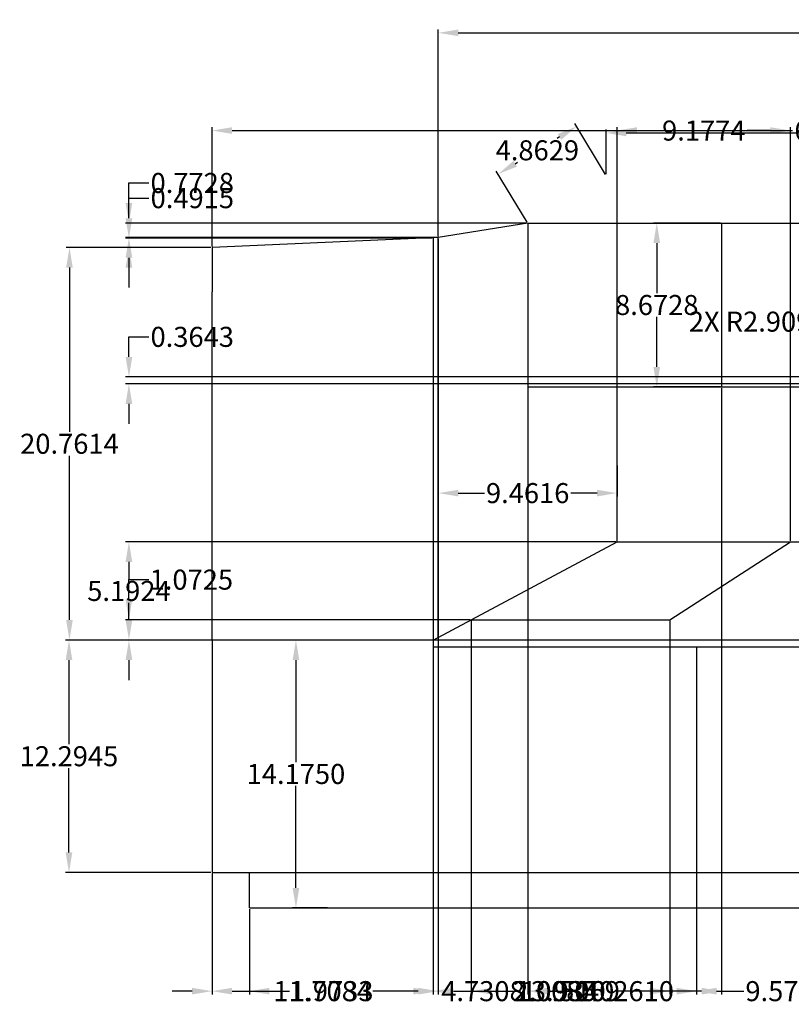
# Model space of a CAD drawing. Units: inches. Extents: x 32.3 to 119.3, y 11.9 to 64.
# Tile 1 of 3: x 32.3 to 73.2, y 11.9 to 64. Entities that reach past the tile are written whole.
import ezdxf

# ---------------------------------------------------------------- set-up
doc = ezdxf.new("R2010")
doc.units = ezdxf.units.IN
doc.header["$MEASUREMENT"] = 0
doc.layers.add('A-ANNO-DIMS', color=2, linetype='Continuous', lineweight=18)
doc.layers.add('A-FURN', color=7, linetype='Continuous', lineweight=25)
doc.styles.get("Standard").update_dxf_attribs({"font": 'arial.ttf'})
doc.dimstyles.get("Standard").update_dxf_attribs({"dimtxt": 1.06, "dimasz": 1.06, "dimexe": 0.18, "dimexo": 0.0625, "dimgap": 0.09, "dimtad": 0, "dimtih": 1, "dimtoh": 1, "dimdec": 4, "dimzin": 0, "dimdsep": 46, "dimtxsty": 'Standard', "dimcen": 0.09, "dimadec": 0, "dimazin": 0, "dimtfac": 1, "dimtdec": 4, "dimtofl": 0, "dimtmove": 0, "dimatfit": 3, "dimfxl": 1, "dimtolj": 1, "dimtzin": 0, "dimarcsym": 0})

# ---------------------------------------------------------------- blocks, each defined once
blk = doc.blocks.new('*D1')
at = {"layer": 'A-ANNO-DIMS', "color": 0, "lineweight": -2, "transparency": 16777216}
for p, q in [((54.478, 52.49), (54.478, 63.441)), ((55.538, 63.261), (75.596, 63.261)), ((101.097, 63.261), (81.039, 63.261)), ((102.157, 52.49), (102.157, 63.441))]:
    blk.add_line(p, q, dxfattribs=at)
at = {"layer": 'A-ANNO-DIMS', "color": 0, "transparency": 16777216}
for points in [[(55.538, 63.438), (55.538, 63.085), (54.478, 63.261)], [(101.097, 63.438), (101.097, 63.085), (102.157, 63.261)]]:
    blk.add_solid(points, dxfattribs=at)
at = {"layer": 'Defpoints', "color": 0, "transparency": 16777216}
for p in [(102.157, 63.261), (54.478, 52.427), (102.157, 52.427)]:
    blk.add_point(p, dxfattribs=at)
at = {"layer": 'A-ANNO-DIMS', "color": 0, "transparency": 16777216, "insert": (78.318, 63.261), "char_height": 1.06, "attachment_point": 5}
blk.add_mtext('\\A1;47.6790', dxfattribs=at)
blk = doc.blocks.new('*D2')
at = {"layer": 'A-ANNO-DIMS', "color": 0, "lineweight": -2, "transparency": 16777216}
for p, q in [((69.408, 53.2), (65.862, 53.2)), ((66.042, 52.14), (66.042, 49.495)), ((66.042, 45.587), (66.042, 48.232)), ((69.408, 44.527), (65.862, 44.527))]:
    blk.add_line(p, q, dxfattribs=at)
at = {"layer": 'A-ANNO-DIMS', "color": 0, "transparency": 16777216}
for points in [[(65.866, 52.14), (66.219, 52.14), (66.042, 53.2)], [(65.866, 45.587), (66.219, 45.587), (66.042, 44.527)]]:
    blk.add_solid(points, dxfattribs=at)
at = {"layer": 'Defpoints', "color": 0, "transparency": 16777216}
for p in [(69.47, 53.2), (66.042, 44.527), (69.47, 44.527)]:
    blk.add_point(p, dxfattribs=at)
at = {"layer": 'A-ANNO-DIMS', "color": 0, "transparency": 16777216, "insert": (66.042, 48.864), "char_height": 1.06, "attachment_point": 5}
blk.add_mtext('\\A1;8.6728', dxfattribs=at)
blk = doc.blocks.new('*D3')
at = {"layer": 'A-ANNO-DIMS', "color": 0, "lineweight": -2, "transparency": 16777216}
for p, q in [((63.336, 55.773), (61.708, 58.461)), ((60.894, 57.758), (60.763, 57.678)), ((58.548, 56.336), (58.679, 56.416)), ((59.177, 53.254), (57.548, 55.941))]:
    blk.add_line(p, q, dxfattribs=at)
at = {"layer": 'A-ANNO-DIMS', "color": 0, "transparency": 16777216}
for points in [[(60.803, 57.909), (60.986, 57.607), (61.801, 58.307)], [(58.457, 56.487), (58.64, 56.185), (57.642, 55.787)]]:
    blk.add_solid(points, dxfattribs=at)
at = {"layer": 'Defpoints', "color": 0, "transparency": 16777216}
for p in [(61.801, 58.307), (63.368, 55.72), (59.209, 53.2)]:
    blk.add_point(p, dxfattribs=at)
at = {"layer": 'A-ANNO-DIMS', "color": 0, "transparency": 16777216, "insert": (59.721, 57.047), "char_height": 1.06, "attachment_point": 5}
blk.add_mtext('\\A1;4.8629', dxfattribs=at)
blk = doc.blocks.new('*D4')
at = {"layer": 'A-ANNO-DIMS', "color": 0, "lineweight": -2, "transparency": 16777216}
for p, q in [((63.368, 55.782), (63.368, 58.146)), ((64.428, 57.966), (80.163, 57.966)), ((101.097, 57.966), (85.362, 57.966)), ((102.157, 55.782), (102.157, 58.146))]:
    blk.add_line(p, q, dxfattribs=at)
at = {"layer": 'A-ANNO-DIMS', "color": 0, "transparency": 16777216}
for points in [[(64.428, 58.142), (64.428, 57.789), (63.368, 57.966)], [(101.097, 58.142), (101.097, 57.789), (102.157, 57.966)]]:
    blk.add_solid(points, dxfattribs=at)
at = {"layer": 'Defpoints', "color": 0, "transparency": 16777216}
for p in [(102.157, 57.966), (63.368, 55.72), (102.157, 55.72)]:
    blk.add_point(p, dxfattribs=at)
at = {"layer": 'A-ANNO-DIMS', "color": 0, "transparency": 16777216, "insert": (82.763, 57.966), "char_height": 1.06, "attachment_point": 5}
blk.add_mtext('\\A1;38.7891', dxfattribs=at)
blk = doc.blocks.new('*D5')
at = {"layer": 'A-ANNO-DIMS', "color": 0, "lineweight": -2, "transparency": 16777216}
for p, q in [((42.445, 51.905), (34.78, 51.905)), ((34.96, 50.845), (34.96, 42.155)), ((34.96, 32.203), (34.96, 40.893)), ((42.445, 31.143), (34.78, 31.143))]:
    blk.add_line(p, q, dxfattribs=at)
at = {"layer": 'A-ANNO-DIMS', "color": 0, "transparency": 16777216}
for points in [[(34.783, 50.845), (35.136, 50.845), (34.96, 51.905)], [(34.783, 32.203), (35.136, 32.203), (34.96, 31.143)]]:
    blk.add_solid(points, dxfattribs=at)
at = {"layer": 'Defpoints', "color": 0, "transparency": 16777216}
for p in [(42.508, 51.905), (34.96, 31.143), (42.508, 31.143)]:
    blk.add_point(p, dxfattribs=at)
at = {"layer": 'A-ANNO-DIMS', "color": 0, "transparency": 16777216, "insert": (34.96, 41.524), "char_height": 1.06, "attachment_point": 5}
blk.add_mtext('\\A1;20.7614', dxfattribs=at)
blk = doc.blocks.new('*D6')
at = {"layer": 'A-ANNO-DIMS', "color": 0, "lineweight": -2, "transparency": 16777216}
for p, q in [((42.445, 31.143), (34.755, 31.143)), ((34.935, 30.083), (34.935, 25.627)), ((34.935, 19.909), (34.935, 24.365)), ((42.445, 18.849), (34.755, 18.849))]:
    blk.add_line(p, q, dxfattribs=at)
at = {"layer": 'A-ANNO-DIMS', "color": 0, "transparency": 16777216}
for points in [[(34.758, 30.083), (35.112, 30.083), (34.935, 31.143)], [(34.758, 19.909), (35.112, 19.909), (34.935, 18.849)]]:
    blk.add_solid(points, dxfattribs=at)
at = {"layer": 'Defpoints', "color": 0, "transparency": 16777216}
for p in [(42.508, 31.143), (34.935, 18.849), (42.508, 18.849)]:
    blk.add_point(p, dxfattribs=at)
at = {"layer": 'A-ANNO-DIMS', "color": 0, "transparency": 16777216, "insert": (34.935, 24.996), "char_height": 1.06, "attachment_point": 5}
blk.add_mtext('\\A1;12.2945', dxfattribs=at)
blk = doc.blocks.new('*D7')
at = {"layer": 'A-ANNO-DIMS', "color": 0, "lineweight": -2, "transparency": 16777216}
for p, q in [((48.3, 31.143), (46.767, 31.143)), ((46.947, 30.083), (46.947, 24.687)), ((46.947, 18.028), (46.947, 23.424)), ((48.62, 16.968), (46.767, 16.968))]:
    blk.add_line(p, q, dxfattribs=at)
at = {"layer": 'A-ANNO-DIMS', "color": 0, "transparency": 16777216}
for points in [[(46.77, 30.083), (47.124, 30.083), (46.947, 31.143)], [(46.77, 18.028), (47.124, 18.028), (46.947, 16.968)]]:
    blk.add_solid(points, dxfattribs=at)
at = {"layer": 'Defpoints', "color": 0, "transparency": 16777216}
for p in [(48.362, 31.143), (46.947, 16.968), (48.683, 16.968)]:
    blk.add_point(p, dxfattribs=at)
at = {"layer": 'A-ANNO-DIMS', "color": 0, "transparency": 16777216, "insert": (46.947, 24.056), "char_height": 1.06, "attachment_point": 5}
blk.add_mtext('\\A1;14.1750', dxfattribs=at)
blk = doc.blocks.new('*D9')
at = {"layer": 'A-ANNO-DIMS', "color": 0, "lineweight": -2, "transparency": 16777216}
for p, q in [((54.478, 40.369), (54.478, 38.734)), ((63.94, 40.369), (63.94, 38.734)), ((55.538, 38.914), (56.919, 38.914)), ((62.88, 38.914), (61.499, 38.914))]:
    blk.add_line(p, q, dxfattribs=at)
at = {"layer": 'A-ANNO-DIMS', "color": 0, "transparency": 16777216}
for points in [[(55.538, 39.091), (55.538, 38.737), (54.478, 38.914)], [(62.88, 39.091), (62.88, 38.737), (63.94, 38.914)]]:
    blk.add_solid(points, dxfattribs=at)
at = {"layer": 'Defpoints', "color": 0, "transparency": 16777216}
for p in [(54.478, 40.431), (63.94, 40.431), (54.478, 38.914)]:
    blk.add_point(p, dxfattribs=at)
at = {"layer": 'A-ANNO-DIMS', "color": 0, "transparency": 16777216, "insert": (59.209, 38.914), "char_height": 1.06, "attachment_point": 5}
blk.add_mtext('\\A1;9.4616', dxfattribs=at)
blk = doc.blocks.new('*D12')
at = {"layer": 'A-ANNO-DIMS', "color": 0, "lineweight": -2, "transparency": 16777216}
for p, q in [((42.508, 51.967), (42.508, 58.272)), ((43.568, 58.092), (73.222, 58.092)), ((108.294, 58.092), (78.64, 58.092)), ((109.354, 36.398), (109.354, 58.272))]:
    blk.add_line(p, q, dxfattribs=at)
at = {"layer": 'A-ANNO-DIMS', "color": 0, "transparency": 16777216}
for points in [[(43.568, 58.269), (43.568, 57.916), (42.508, 58.092)], [(108.294, 58.269), (108.294, 57.916), (109.354, 58.092)]]:
    blk.add_solid(points, dxfattribs=at)
at = {"layer": 'Defpoints', "color": 0, "transparency": 16777216}
for p in [(109.354, 58.092), (42.508, 51.905), (109.354, 36.335)]:
    blk.add_point(p, dxfattribs=at)
at = {"layer": 'A-ANNO-DIMS', "color": 0, "transparency": 16777216, "insert": (75.931, 58.092), "char_height": 1.06, "attachment_point": 5}
blk.add_mtext('\\A1;66.8465', dxfattribs=at)
blk = doc.blocks.new('*D13')
at = {"layer": 'A-ANNO-DIMS', "color": 0, "lineweight": -2, "transparency": 16777216}
for p, q in [((42.508, 18.786), (42.508, 12.388)), ((44.481, 16.906), (44.481, 12.388)), ((41.448, 12.568), (40.388, 12.568)), ((45.541, 12.568), (46.601, 12.568))]:
    blk.add_line(p, q, dxfattribs=at)
at = {"layer": 'A-ANNO-DIMS', "color": 0, "transparency": 16777216}
for points in [[(41.448, 12.745), (41.448, 12.391), (42.508, 12.568)], [(45.541, 12.745), (45.541, 12.391), (44.481, 12.568)]]:
    blk.add_solid(points, dxfattribs=at)
at = {"layer": 'Defpoints', "color": 0, "transparency": 16777216}
for p in [(42.508, 18.849), (44.481, 16.968), (44.481, 12.568)]:
    blk.add_point(p, dxfattribs=at)
at = {"layer": 'A-ANNO-DIMS', "color": 0, "transparency": 16777216, "insert": (48.842, 12.568), "char_height": 1.06, "attachment_point": 5}
blk.add_mtext('\\A1;1.9733', dxfattribs=at)
blk = doc.blocks.new('*D14')
at = {"layer": 'A-ANNO-DIMS', "color": 0, "lineweight": -2, "transparency": 16777216}
for p, q in [((42.508, 18.786), (42.508, 12.388)), ((54.216, 18.786), (54.216, 12.388)), ((43.568, 12.568), (45.712, 12.568)), ((53.156, 12.568), (51.012, 12.568))]:
    blk.add_line(p, q, dxfattribs=at)
at = {"layer": 'A-ANNO-DIMS', "color": 0, "transparency": 16777216}
for points in [[(43.568, 12.745), (43.568, 12.391), (42.508, 12.568)], [(53.156, 12.745), (53.156, 12.391), (54.216, 12.568)]]:
    blk.add_solid(points, dxfattribs=at)
at = {"layer": 'Defpoints', "color": 0, "transparency": 16777216}
for p in [(42.508, 18.849), (54.216, 18.849), (54.216, 12.568)]:
    blk.add_point(p, dxfattribs=at)
at = {"layer": 'A-ANNO-DIMS', "color": 0, "transparency": 16777216, "insert": (48.362, 12.568), "char_height": 1.06, "attachment_point": 5}
blk.add_mtext('\\A1;11.7084', dxfattribs=at)
blk = doc.blocks.new('*D15')
at = {"layer": 'A-ANNO-DIMS', "color": 0, "lineweight": -2, "transparency": 16777216}
for p, q in [((54.216, 18.786), (54.216, 12.388)), ((68.15, 18.786), (68.15, 12.388)), ((55.276, 12.568), (58.533, 12.568)), ((67.09, 12.568), (63.834, 12.568))]:
    blk.add_line(p, q, dxfattribs=at)
at = {"layer": 'A-ANNO-DIMS', "color": 0, "transparency": 16777216}
for points in [[(55.276, 12.745), (55.276, 12.391), (54.216, 12.568)], [(67.09, 12.745), (67.09, 12.391), (68.15, 12.568)]]:
    blk.add_solid(points, dxfattribs=at)
at = {"layer": 'Defpoints', "color": 0, "transparency": 16777216}
for p in [(54.216, 18.849), (68.15, 18.849), (68.15, 12.568)]:
    blk.add_point(p, dxfattribs=at)
at = {"layer": 'A-ANNO-DIMS', "color": 0, "transparency": 16777216, "insert": (61.183, 12.568), "char_height": 1.06, "attachment_point": 5}
blk.add_mtext('\\A1;13.9340', dxfattribs=at)
blk = doc.blocks.new('*D16')
at = {"layer": 'A-ANNO-DIMS', "color": 0, "lineweight": -2, "transparency": 16777216}
for p, q in [((77.726, 21.181), (77.726, 12.388)), ((68.15, 18.786), (68.15, 12.388)), ((69.21, 12.568), (70.647, 12.568)), ((76.666, 12.568), (75.23, 12.568))]:
    blk.add_line(p, q, dxfattribs=at)
at = {"layer": 'A-ANNO-DIMS', "color": 0, "transparency": 16777216}
for points in [[(69.21, 12.745), (69.21, 12.391), (68.15, 12.568)], [(76.666, 12.745), (76.666, 12.391), (77.726, 12.568)]]:
    blk.add_solid(points, dxfattribs=at)
at = {"layer": 'Defpoints', "color": 0, "transparency": 16777216}
for p in [(77.726, 21.244), (68.15, 18.849), (77.726, 12.568)]:
    blk.add_point(p, dxfattribs=at)
at = {"layer": 'A-ANNO-DIMS', "color": 0, "transparency": 16777216, "insert": (72.938, 12.568), "char_height": 1.06, "attachment_point": 5}
blk.add_mtext('\\A1;9.5758', dxfattribs=at)
blk = doc.blocks.new('*D24')
at = {"layer": 'A-ANNO-DIMS', "color": 0, "lineweight": -2, "transparency": 16777216}
for p, q in [((59.209, 53.138), (59.209, 12.388)), ((54.478, 52.365), (54.478, 12.388)), ((53.418, 12.568), (52.358, 12.568)), ((60.269, 12.568), (61.329, 12.568))]:
    blk.add_line(p, q, dxfattribs=at)
at = {"layer": 'A-ANNO-DIMS', "color": 0, "transparency": 16777216}
for points in [[(53.418, 12.745), (53.418, 12.391), (54.478, 12.568)], [(60.269, 12.745), (60.269, 12.391), (59.209, 12.568)]]:
    blk.add_solid(points, dxfattribs=at)
at = {"layer": 'Defpoints', "color": 0, "transparency": 16777216}
for p in [(59.209, 53.2), (54.478, 52.427), (59.209, 12.568)]:
    blk.add_point(p, dxfattribs=at)
at = {"layer": 'A-ANNO-DIMS', "color": 0, "transparency": 16777216, "insert": (56.844, 12.568), "char_height": 1.06, "attachment_point": 5}
blk.add_mtext('\\A1;4.7308', dxfattribs=at)
blk = doc.blocks.new('*D25')
at = {"layer": 'A-ANNO-DIMS', "color": 0, "lineweight": -2, "transparency": 16777216}
for p, q in [((59.209, 44.465), (59.209, 12.388)), ((69.47, 44.465), (69.47, 12.388)), ((60.269, 12.568), (61.689, 12.568)), ((68.41, 12.568), (66.99, 12.568))]:
    blk.add_line(p, q, dxfattribs=at)
at = {"layer": 'A-ANNO-DIMS', "color": 0, "transparency": 16777216}
for points in [[(60.269, 12.745), (60.269, 12.391), (59.209, 12.568)], [(68.41, 12.745), (68.41, 12.391), (69.47, 12.568)]]:
    blk.add_solid(points, dxfattribs=at)
at = {"layer": 'Defpoints', "color": 0, "transparency": 16777216}
for p in [(59.209, 44.527), (69.47, 44.527), (69.47, 12.568)]:
    blk.add_point(p, dxfattribs=at)
at = {"layer": 'A-ANNO-DIMS', "color": 0, "transparency": 16777216, "insert": (64.34, 12.568), "char_height": 1.06, "attachment_point": 5}
blk.add_mtext('\\A1;10.2610', dxfattribs=at)
blk = doc.blocks.new('*D31')
at = {"layer": 'A-ANNO-DIMS', "color": 0, "lineweight": -2, "transparency": 16777216}
for p, q in [((38.108, 54.26), (38.108, 55.32)), ((38.108, 55.32), (39.168, 55.32)), ((59.147, 53.2), (37.928, 53.2)), ((54.416, 52.427), (37.928, 52.427)), ((38.108, 51.367), (38.108, 50.307))]:
    blk.add_line(p, q, dxfattribs=at)
at = {"layer": 'A-ANNO-DIMS', "color": 0, "transparency": 16777216}
for points in [[(37.931, 54.26), (38.285, 54.26), (38.108, 53.2)], [(37.931, 51.367), (38.285, 51.367), (38.108, 52.427)]]:
    blk.add_solid(points, dxfattribs=at)
at = {"layer": 'Defpoints', "color": 0, "transparency": 16777216}
for p in [(38.108, 53.2), (59.209, 53.2), (54.478, 52.427)]:
    blk.add_point(p, dxfattribs=at)
at = {"layer": 'A-ANNO-DIMS', "color": 0, "transparency": 16777216, "insert": (41.459, 55.32), "char_height": 1.06, "attachment_point": 5}
blk.add_mtext('\\A1;0.7728', dxfattribs=at)
blk = doc.blocks.new('*D32')
at = {"layer": 'A-ANNO-DIMS', "color": 0, "lineweight": -2, "transparency": 16777216}
for p, q in [((38.108, 53.456), (38.108, 54.516)), ((38.108, 54.516), (39.168, 54.516)), ((54.154, 52.396), (37.928, 52.396)), ((42.445, 51.905), (37.928, 51.905)), ((38.108, 50.845), (38.108, 49.785))]:
    blk.add_line(p, q, dxfattribs=at)
at = {"layer": 'A-ANNO-DIMS', "color": 0, "transparency": 16777216}
for points in [[(37.931, 53.456), (38.285, 53.456), (38.108, 52.396)], [(37.931, 50.845), (38.285, 50.845), (38.108, 51.905)]]:
    blk.add_solid(points, dxfattribs=at)
at = {"layer": 'Defpoints', "color": 0, "transparency": 16777216}
for p in [(38.108, 52.396), (54.216, 52.396), (42.508, 51.905)]:
    blk.add_point(p, dxfattribs=at)
at = {"layer": 'A-ANNO-DIMS', "color": 0, "transparency": 16777216, "insert": (41.462, 54.516), "char_height": 1.06, "attachment_point": 5}
blk.add_mtext('\\A1;0.4915', dxfattribs=at)
blk = doc.blocks.new('*D40')
at = {"layer": 'A-ANNO-DIMS', "color": 0, "lineweight": -2, "transparency": 16777216}
for p, q in [((38.108, 46.119), (38.108, 47.179)), ((38.108, 47.179), (39.168, 47.179)), ((80.758, 45.059), (37.928, 45.059)), ((80.758, 44.694), (37.928, 44.694)), ((38.108, 43.634), (38.108, 42.574))]:
    blk.add_line(p, q, dxfattribs=at)
at = {"layer": 'A-ANNO-DIMS', "color": 0, "transparency": 16777216}
for points in [[(37.931, 46.119), (38.285, 46.119), (38.108, 45.059)], [(37.931, 43.634), (38.285, 43.634), (38.108, 44.694)]]:
    blk.add_solid(points, dxfattribs=at)
at = {"layer": 'Defpoints', "color": 0, "transparency": 16777216}
for p in [(38.108, 45.059), (80.821, 45.059), (80.821, 44.694)]:
    blk.add_point(p, dxfattribs=at)
at = {"layer": 'A-ANNO-DIMS', "color": 0, "transparency": 16777216, "insert": (41.458, 47.179), "char_height": 1.06, "attachment_point": 5}
blk.add_mtext('\\A1;0.3643', dxfattribs=at)
blk = doc.blocks.new('*D41')
at = {"layer": 'A-ANNO-DIMS', "color": 0, "lineweight": -2, "transparency": 16777216}
for p, q in [((56.225, 32.153), (56.225, 12.388)), ((54.216, 31.081), (54.216, 12.388)), ((53.156, 12.568), (52.096, 12.568)), ((57.285, 12.568), (58.345, 12.568))]:
    blk.add_line(p, q, dxfattribs=at)
at = {"layer": 'A-ANNO-DIMS', "color": 0, "transparency": 16777216}
for points in [[(53.156, 12.745), (53.156, 12.391), (54.216, 12.568)], [(57.285, 12.745), (57.285, 12.391), (56.225, 12.568)]]:
    blk.add_solid(points, dxfattribs=at)
at = {"layer": 'Defpoints', "color": 0, "transparency": 16777216}
for p in [(56.225, 32.216), (54.216, 31.143), (56.225, 12.568)]:
    blk.add_point(p, dxfattribs=at)
at = {"layer": 'A-ANNO-DIMS', "color": 0, "transparency": 16777216, "insert": (60.648, 12.568), "char_height": 1.06, "attachment_point": 5}
blk.add_mtext('\\A1;2.0085', dxfattribs=at)
blk = doc.blocks.new('*D42')
at = {"layer": 'A-ANNO-DIMS', "color": 0, "lineweight": -2, "transparency": 16777216}
for p, q in [((56.225, 32.153), (56.225, 12.388)), ((66.732, 32.153), (66.732, 12.388)), ((57.285, 12.568), (58.825, 12.568)), ((65.672, 12.568), (64.132, 12.568))]:
    blk.add_line(p, q, dxfattribs=at)
at = {"layer": 'A-ANNO-DIMS', "color": 0, "transparency": 16777216}
for points in [[(57.285, 12.745), (57.285, 12.391), (56.225, 12.568)], [(65.672, 12.745), (65.672, 12.391), (66.732, 12.568)]]:
    blk.add_solid(points, dxfattribs=at)
at = {"layer": 'Defpoints', "color": 0, "transparency": 16777216}
for p in [(56.225, 32.216), (66.732, 32.216), (66.732, 12.568)]:
    blk.add_point(p, dxfattribs=at)
at = {"layer": 'A-ANNO-DIMS', "color": 0, "transparency": 16777216, "insert": (61.478, 12.568), "char_height": 1.06, "attachment_point": 5}
blk.add_mtext('\\A1;10.5069', dxfattribs=at)
blk = doc.blocks.new('*D43')
at = {"layer": 'A-ANNO-DIMS', "color": 0, "lineweight": -2, "transparency": 16777216}
for p, q in [((38.108, 33.276), (38.108, 34.336)), ((38.108, 34.336), (39.168, 34.336)), ((56.162, 32.216), (37.928, 32.216)), ((54.154, 31.143), (37.928, 31.143)), ((38.108, 30.083), (38.108, 29.023))]:
    blk.add_line(p, q, dxfattribs=at)
at = {"layer": 'A-ANNO-DIMS', "color": 0, "transparency": 16777216}
for points in [[(37.931, 33.276), (38.285, 33.276), (38.108, 32.216)], [(37.931, 30.083), (38.285, 30.083), (38.108, 31.143)]]:
    blk.add_solid(points, dxfattribs=at)
at = {"layer": 'Defpoints', "color": 0, "transparency": 16777216}
for p in [(38.108, 32.216), (56.225, 32.216), (54.216, 31.143)]:
    blk.add_point(p, dxfattribs=at)
at = {"layer": 'A-ANNO-DIMS', "color": 0, "transparency": 16777216, "insert": (41.412, 34.336), "char_height": 1.06, "attachment_point": 5}
blk.add_mtext('\\A1;1.0725', dxfattribs=at)
blk = doc.blocks.new('*D44')
at = {"layer": 'A-ANNO-DIMS', "color": 0, "lineweight": -2, "transparency": 16777216}
for p, q in [((63.94, 36.398), (63.94, 58.272)), ((65, 58.092), (66.24, 58.092)), ((72.057, 58.092), (70.817, 58.092)), ((73.117, 36.398), (73.117, 58.272))]:
    blk.add_line(p, q, dxfattribs=at)
at = {"layer": 'A-ANNO-DIMS', "color": 0, "transparency": 16777216}
for points in [[(65, 58.269), (65, 57.916), (63.94, 58.092)], [(72.057, 58.269), (72.057, 57.916), (73.117, 58.092)]]:
    blk.add_solid(points, dxfattribs=at)
at = {"layer": 'Defpoints', "color": 0, "transparency": 16777216}
for p in [(73.117, 58.092), (63.94, 36.335), (73.117, 36.335)]:
    blk.add_point(p, dxfattribs=at)
at = {"layer": 'A-ANNO-DIMS', "color": 0, "transparency": 16777216, "insert": (68.529, 58.092), "char_height": 1.06, "attachment_point": 5}
blk.add_mtext('\\A1;9.1774', dxfattribs=at)
blk = doc.blocks.new('*D51')
at = {"layer": 'A-ANNO-DIMS', "color": 0, "lineweight": -2, "transparency": 16777216}
for p, q in [((63.877, 36.335), (37.928, 36.335)), ((38.108, 35.275), (38.108, 34.37)), ((38.108, 32.203), (38.108, 33.108)), ((54.154, 31.143), (37.928, 31.143))]:
    blk.add_line(p, q, dxfattribs=at)
at = {"layer": 'A-ANNO-DIMS', "color": 0, "transparency": 16777216}
for points in [[(37.931, 35.275), (38.285, 35.275), (38.108, 36.335)], [(37.931, 32.203), (38.285, 32.203), (38.108, 31.143)]]:
    blk.add_solid(points, dxfattribs=at)
at = {"layer": 'Defpoints', "color": 0, "transparency": 16777216}
for p in [(38.108, 36.335), (63.94, 36.335), (54.216, 31.143)]:
    blk.add_point(p, dxfattribs=at)
at = {"layer": 'A-ANNO-DIMS', "color": 0, "transparency": 16777216, "insert": (38.108, 33.739), "char_height": 1.06, "attachment_point": 5}
blk.add_mtext('\\A1;5.1924', dxfattribs=at)
blk = doc.blocks.new('*D61')
at = {"layer": 'A-ANNO-DIMS', "color": 0, "lineweight": -2, "transparency": 16777216}
for p, q in [((75.325, 47.985), (76.385, 47.985)), ((76.385, 47.985), (77.19, 47.295)), ((80.202, 44.62), (80.202, 44.8)), ((80.112, 44.71), (80.292, 44.71))]:
    blk.add_line(p, q, dxfattribs=at)
at = {"layer": 'A-ANNO-DIMS', "color": 0, "transparency": 16777216}
blk.add_solid([(77.305, 47.429), (77.075, 47.161), (77.994, 46.605)], dxfattribs=at)
at = {"layer": 'Defpoints', "color": 0, "transparency": 16777216}
for p in [(77.994, 46.605), (80.202, 44.71)]:
    blk.add_point(p, dxfattribs=at)
at = {"layer": 'A-ANNO-DIMS', "color": 0, "transparency": 16777216, "insert": (71.38, 47.985), "char_height": 1.06, "attachment_point": 5}
blk.add_mtext('\\A1;2X R2.9096', dxfattribs=at)

msp = doc.modelspace()

# ---------------------------------------------------------------- linework, layer by layer
at = {"layer": 'A-FURN'}
for p, q in [((59.20908, 53.20007), (54.4783, 52.42729)), ((59.20908, 53.20007), (59.20908, 44.52731)), ((59.20908, 53.20007), (99.43717, 53.20007)), ((69.47003, 53.20007), (69.47003, 44.52731)), ((54.4783, 52.42729), (42.50795, 51.90451)), ((54.2164, 52.39602), (54.2164, 18.84862)), ((54.4783, 31.28294), (54.4783, 52.42729)), ((42.50795, 51.90451), (42.50795, 49.56661)), ((42.50795, 31.14308), (42.50795, 49.56661)), ((59.20908, 44.52731), (99.43717, 44.52731)), ((63.93986, 36.33549), (63.93986, 44.52731)), ((54.2164, 31.14308), (63.93986, 36.33549)), ((63.93986, 36.33549), (109.35445, 36.33549)), ((66.73172, 32.21562), (73.11726, 36.33549)), ((56.22486, 32.21562), (66.73172, 32.21562)), ((42.50795, 31.14308), (42.50795, 18.84862)), ((54.2164, 31.14308), (42.50795, 31.14308)), ((99.63098, 31.14308), (54.2164, 31.14308)), ((99.63098, 30.76852), (54.2164, 30.76852)), ((68.15041, 30.76852), (68.15041, 18.84862)), ((42.50795, 18.84862), (99.66402, 18.84862)), ((44.48125, 16.9681), (44.48125, 18.84862)), ((44.48125, 16.9681), (54.2164, 16.9681)), ((54.2164, 16.9681), (99.63098, 16.9681))]:
    msp.add_line(p, q, dxfattribs=at)

# ---------------------------------------------------------------- dimensions: what is measured, and where the dimension line sits
at = {"layer": 'A-ANNO-DIMS'}
for base, p1, p2, override, picture, middle in [((102.15728, 63.26132), (54.4783, 52.42729), (102.15728, 52.42729), {"dimclrd": 0, "dimclre": 0, "dimclrt": 0}, '*D1', (78.31779, 63.26132)), ((109.35445, 58.09249), (42.50795, 51.90451), (109.35445, 36.33549), {"dimdec": 4, "dimlfac": 1, "dimrnd": 0, "dimzin": 0, "dimdsep": 46, "dimlunit": 2}, '*D12', (75.9312, 58.09249)), ((102.15728, 57.96555), (63.36818, 55.71994), (102.15728, 55.71994), {"dimclrd": 0, "dimclre": 0, "dimclrt": 0}, '*D4', (82.76273, 57.96555)), ((73.11727, 58.09249), (63.93986, 36.33549), (73.11727, 36.33549), {"dimdec": 4, "dimlfac": 1, "dimrnd": 0, "dimzin": 0, "dimdsep": 46, "dimlunit": 2}, '*D44', (68.52856, 58.09249)), ((59.20908, 12.5681), (54.4783, 52.42729), (59.20908, 53.20007), {"dimdec": 4, "dimlfac": 1, "dimrnd": 0, "dimzin": 0, "dimdsep": 46, "dimlunit": 2}, '*D24', (56.84369, 12.5681)), ((69.470031, 12.5681), (59.209079, 44.527306), (69.470031, 44.527306), {"dimdec": 4, "dimlfac": 1, "dimrnd": 0, "dimzin": 0, "dimdsep": 46, "dimlunit": 2}, '*D25', (64.339555, 12.5681)), ((54.4783, 38.91411), (63.93986, 40.4314), (54.4783, 40.4314), {"dimclrd": 0, "dimclre": 0, "dimclrt": 0}, '*D9', (59.20908, 38.91411)), ((56.22486, 12.5681), (54.2164, 31.14308), (56.22486, 32.21562), {"dimdec": 4, "dimlfac": 1, "dimrnd": 0, "dimzin": 0, "dimdsep": 46, "dimlunit": 2}, '*D41', (60.64814, 12.5681)), ((66.73172, 12.5681), (56.22486, 32.21562), (66.73172, 32.21562), {"dimdec": 4, "dimlfac": 1, "dimrnd": 0, "dimzin": 0, "dimdsep": 46, "dimlunit": 2}, '*D42', (61.47829, 12.5681)), ((77.72624, 12.5681), (68.15041, 18.84862), (77.72624, 21.24379), {"dimdec": 4, "dimlfac": 1, "dimrnd": 0, "dimzin": 0, "dimdsep": 46, "dimlunit": 2}, '*D16', (72.93832, 12.5681)), ((44.48125, 12.5681), (42.50795, 18.84862), (44.48125, 16.9681), {"dimdec": 4, "dimlfac": 1, "dimrnd": 0, "dimzin": 0, "dimdsep": 46, "dimlunit": 2}, '*D13', (48.84162, 12.5681)), ((54.216398, 12.5681), (42.507951, 18.848621), (54.216398, 18.848621), {"dimdec": 4, "dimlfac": 1, "dimrnd": 0, "dimzin": 0, "dimdsep": 46, "dimlunit": 2}, '*D14', (48.362174, 12.5681)), ((68.15041, 12.5681), (54.2164, 18.84862), (68.15041, 18.84862), {"dimdec": 4, "dimlfac": 1, "dimrnd": 0, "dimzin": 0, "dimdsep": 46, "dimlunit": 2}, '*D15', (61.1834, 12.5681))]:
    dim = msp.add_linear_dim(base=base, p1=p1, p2=p2, dimstyle='Standard', override=override, dxfattribs=at)
    dim.commit()
    dim.dimension.update_dxf_attribs({"geometry": picture, "text_midpoint": middle})
dim = msp.add_aligned_dim(p1=(59.20908, 53.20007), p2=(63.36818, 55.71994), distance=3.0247, dimstyle='Standard', override={"dimclrd": 0, "dimclre": 0, "dimclrt": 0}, dxfattribs=at)
dim.commit()
dim.dimension.update_dxf_attribs({"geometry": '*D3', "text_midpoint": (59.72128, 57.04694)})
for base, p1, p2, override, picture, middle in [((38.10795, 53.20007), (54.4783, 52.42729), (59.20908, 53.20007), {"dimdec": 4, "dimlfac": 1, "dimrnd": 0, "dimzin": 0, "dimdsep": 46, "dimlunit": 2}, '*D31', (41.45929, 55.32007)), ((38.10795, 52.39602), (42.50795, 51.90451), (54.2164, 52.39602), {"dimdec": 4, "dimlfac": 1, "dimrnd": 0, "dimzin": 0, "dimdsep": 46, "dimlunit": 2}, '*D32', (41.46219, 54.51602)), ((66.04232, 44.52731), (69.47003, 53.20007), (69.47003, 44.52731), {"dimclrd": 0, "dimclre": 0, "dimclrt": 0}, '*D2', (66.04232, 48.86369)), ((34.95975, 31.14308), (42.50795, 51.90451), (42.50795, 31.14308), {"dimclrd": 0, "dimclre": 0, "dimclrt": 0}, '*D5', (34.95975, 41.5238)), ((38.10795, 45.05867), (80.82094, 44.6944), (80.82094, 45.05867), {"dimdec": 4, "dimlfac": 1, "dimrnd": 0, "dimzin": 0, "dimdsep": 46, "dimlunit": 2}, '*D40', (41.45821, 47.17867)), ((38.10795, 36.33549), (54.2164, 31.14308), (63.93986, 36.33549), {"dimdec": 4, "dimlfac": 1, "dimrnd": 0, "dimzin": 0, "dimdsep": 46, "dimlunit": 2}, '*D51', (38.10795, 33.73929)), ((38.10795, 32.21562), (54.2164, 31.14308), (56.22486, 32.21562), {"dimdec": 4, "dimlfac": 1, "dimrnd": 0, "dimzin": 0, "dimdsep": 46, "dimlunit": 2}, '*D43', (41.4123, 34.33562)), ((34.93489, 18.84862), (42.50795, 31.14308), (42.50795, 18.84862), {"dimclrd": 0, "dimclre": 0, "dimclrt": 0}, '*D6', (34.93489, 24.99585)), ((46.94687, 16.9681), (48.36217, 31.14308), (48.68271, 16.9681), {"dimclrd": 0, "dimclre": 0, "dimclrt": 0}, '*D7', (46.94687, 24.05559))]:
    dim = msp.add_linear_dim(base=base, p1=p1, p2=p2, angle=90, dimstyle='Standard', override=override, dxfattribs=at)
    dim.commit()
    dim.dimension.update_dxf_attribs({"geometry": picture, "text_midpoint": middle})
dim = msp.add_radius_dim(center=(80.20238, 44.71033), mpoint=(77.99423, 46.60495), text='2X <>', dimstyle='Standard', override={"dimdec": 4, "dimlfac": 1, "dimrnd": 0, "dimzin": 0, "dimdsep": 46, "dimlunit": 2}, dxfattribs=at)
dim.commit()
dim.dimension.update_dxf_attribs({"geometry": '*D61', "text_midpoint": (71.38032, 47.98544)})

doc.saveas('drawing.dxf')
